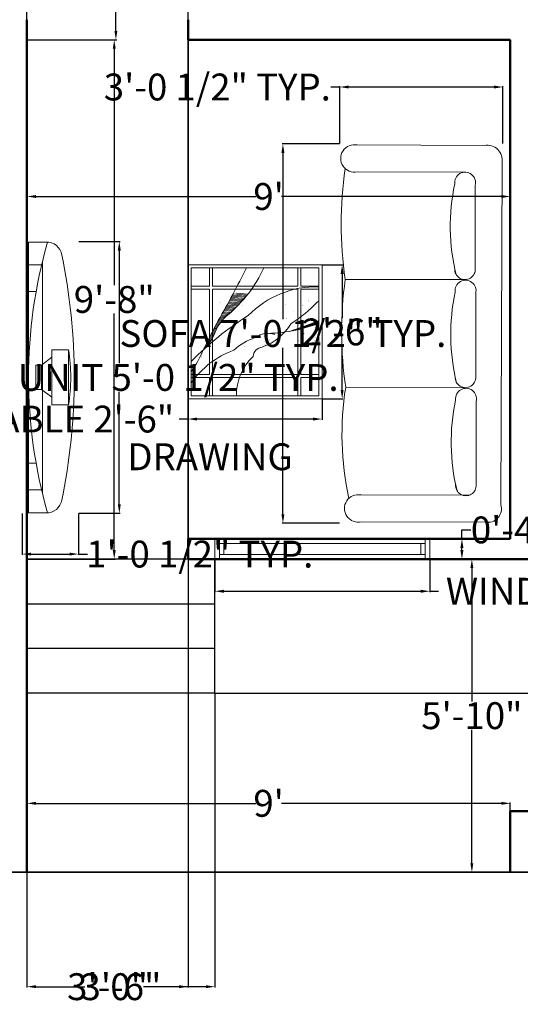
# Model space of a CAD drawing. Units: inches. Extents: x 134 to 568, y 15 to 554.
# Tile 2 of 7: x 303 to 415, y 15 to 235. Entities that reach past the tile are written whole.
import ezdxf

# ---------------------------------------------------------------- set-up
doc = ezdxf.new("R2010")
doc.units = ezdxf.units.IN
doc.header["$MEASUREMENT"] = 0
for name, color, linetype, lineweight in [('A-ANNO-DIMS', 2, 'Continuous', 18), ('A-AREA-IDEN', 7, 'Continuous', 25), ('A-EQPM', 8, 'Continuous', 18), ('A-FLOR-STRS', 3, 'Continuous', 25), ('A-FURN', 9, 'Continuous', 18), ('A-GLAZ', 4, 'Continuous', 18), ('A-WALL', 7, 'Continuous', 50), ('C-PROP', 7, 'Continuous', 35)]:
    doc.layers.add(name, color=color, linetype=linetype, lineweight=lineweight)
doc.styles.get("Standard").update_dxf_attribs({"font": 'arial.ttf'})
doc.dimstyles.get("Standard").update_dxf_attribs({"dimtxt": 6, "dimasz": 2, "dimexe": 0.18, "dimexo": 0.0625, "dimgap": 0.09, "dimtad": 0, "dimtih": 1, "dimtoh": 1, "dimdec": 0, "dimzin": 0, "dimdsep": 46, "dimlunit": 4, "dimtxsty": 'Standard', "dimcen": 0.09, "dimadec": 0, "dimazin": 0, "dimtfac": 1, "dimtdec": 0, "dimtofl": 0, "dimtmove": 0, "dimatfit": 3, "dimfxl": 1, "dimtolj": 1, "dimtzin": 0, "dimarcsym": 0})

# ---------------------------------------------------------------- blocks, each defined once
blk = doc.blocks.new('window 4.5')
for p, q in [((346.5833573093669, -32.94169834523767), (346.5833573093669, -28.44169834523766)), ((346.5833573093669, -28.44169834523766), (394.5833573093669, -28.44169834523766)), ((347.5833573093669, -32.94169834523768), (347.583357309367, -28.44169834523767)), ((393.5833573093669, -28.44169834523766), (393.5833573093669, -32.94169834523766)), ((394.5833573093669, -28.44169834523766), (394.5833573093669, -32.94169834523766)), ((347.5833573093669, -29.44169834523766), (393.5833573093669, -29.44169834523765)), ((348.5833573093669, -31.94169834523767), (348.5833573093669, -29.44169834523765)), ((392.5833573093669, -29.44169834523765), (392.5833573093669, -31.94169834523766)), ((394.5833573093669, -32.94169834523766), (346.5833573093669, -32.94169834523767)), ((393.5833573093669, -31.94169834523766), (347.5833573093669, -31.94169834523767))]:
    blk.add_line(p, q)
blk = doc.blocks.new('*D10')
at = {"layer": 'A-ANNO-DIMS', "color": 0, "lineweight": -2, "transparency": 16777216}
for p, q in [((304.583357309367, 44.64466191446035), (304.583357309367, 60.17594326257374)), ((306.583357309367, 59.99594326257374), (355.7327843216453, 59.99594326257374)), ((410.5833573093669, 59.99594326257374), (361.4339302970887, 59.99594326257374)), ((412.583357309367, 44.64466191446035), (412.583357309367, 60.17594326257374))]:
    blk.add_line(p, q, dxfattribs=at)
at = {"layer": 'A-ANNO-DIMS', "color": 0, "transparency": 16777216}
for points in [[(306.583357309367, 60.32927659590708), (306.583357309367, 59.66260992924041), (304.583357309367, 59.99594326257374)], [(410.5833573093669, 60.32927659590708), (410.5833573093669, 59.66260992924041), (412.583357309367, 59.99594326257374)]]:
    blk.add_solid(points, dxfattribs=at)
at = {"layer": 'Defpoints', "color": 0, "transparency": 16777216}
for p in [(412.583357309367, 59.99594326257374), (304.583357309367, 44.58216191446036), (412.583357309367, 44.58216191446036)]:
    blk.add_point(p, dxfattribs=at)
at = {"layer": 'A-ANNO-DIMS', "color": 0, "transparency": 16777216, "insert": (358.583357309367, 59.99594326257374), "char_height": 6, "attachment_point": 5}
blk.add_mtext("\\A1;9'", dxfattribs=at)
blk = doc.blocks.new('*D11')
at = {"layer": 'A-ANNO-DIMS', "color": 0, "lineweight": -2, "transparency": 16777216}
for p, q in [((417.020857309367, 114.5821619144604), (403.8256208830564, 114.5821619144604)), ((404.0056208830565, 112.5821619144604), (404.0056208830565, 82.73559984079056)), ((404.0056208830565, 46.58216191446037), (404.0056208830565, 76.42872398813023)), ((412.5208573093671, 44.58216191446036), (403.8256208830564, 44.58216191446036))]:
    blk.add_line(p, q, dxfattribs=at)
at = {"layer": 'A-ANNO-DIMS', "color": 0, "transparency": 16777216}
for points in [[(403.6722875497232, 112.5821619144604), (404.3389542163898, 112.5821619144604), (404.0056208830565, 114.5821619144604)], [(403.6722875497232, 46.58216191446037), (404.3389542163898, 46.58216191446037), (404.0056208830565, 44.58216191446036)]]:
    blk.add_solid(points, dxfattribs=at)
at = {"layer": 'Defpoints', "color": 0, "transparency": 16777216}
for p in [(404.0056208830565, 114.5821619144604), (417.0833573093671, 114.5821619144604), (412.5833573093671, 44.58216191446036)]:
    blk.add_point(p, dxfattribs=at)
at = {"layer": 'A-ANNO-DIMS', "color": 0, "transparency": 16777216, "insert": (404.0056208830564, 79.58216191446026), "char_height": 6, "attachment_point": 5}
blk.add_mtext('\\A1;5\'-10"', dxfattribs=at)
blk = doc.blocks.new('*D12')
at = {"layer": 'A-ANNO-DIMS', "color": 0, "lineweight": -2, "transparency": 16777216}
for p, q in [((304.5833573093669, 230.5196619144604), (304.5833573093669, 195.3989397718649)), ((412.5833573093668, 230.5196619144604), (412.5833573093668, 195.3989397718649)), ((306.5833573093669, 195.5789397718649), (355.7327843216452, 195.5789397718649)), ((410.5833573093669, 195.5789397718649), (361.4339302970886, 195.5789397718649))]:
    blk.add_line(p, q, dxfattribs=at)
at = {"layer": 'A-ANNO-DIMS', "color": 0, "transparency": 16777216}
for points in [[(306.5833573093669, 195.9122731051983), (306.5833573093669, 195.2456064385316), (304.5833573093669, 195.5789397718649)], [(410.5833573093669, 195.9122731051983), (410.5833573093669, 195.2456064385316), (412.5833573093668, 195.5789397718649)]]:
    blk.add_solid(points, dxfattribs=at)
at = {"layer": 'Defpoints', "color": 0, "transparency": 16777216}
for p in [(304.5833573093669, 230.5821619144603), (412.5833573093668, 230.5821619144603), (412.5833573093668, 195.5789397718649)]:
    blk.add_point(p, dxfattribs=at)
at = {"layer": 'A-ANNO-DIMS', "color": 0, "transparency": 16777216, "insert": (358.5833573093669, 195.5789397718649), "char_height": 6, "attachment_point": 5}
blk.add_mtext("\\A1;9'", dxfattribs=at)
blk = doc.blocks.new('*D13')
at = {"layer": 'A-ANNO-DIMS', "color": 0, "lineweight": -2, "transparency": 16777216}
for p, q in [((304.6458573093671, 230.5821619144605), (324.2629623244103, 230.5821619144605)), ((324.0829623244104, 228.5821619144605), (324.0829623244104, 175.7355998407906)), ((324.0829623244104, 116.5821619144604), (324.0829623244104, 169.4287239881303)), ((304.6458573093671, 114.5821619144604), (324.2629623244104, 114.5821619144604))]:
    blk.add_line(p, q, dxfattribs=at)
at = {"layer": 'A-ANNO-DIMS', "color": 0, "transparency": 16777216}
for points in [[(323.749628991077, 228.5821619144605), (324.4162956577437, 228.5821619144605), (324.0829623244104, 230.5821619144605)], [(323.7496289910771, 116.5821619144604), (324.4162956577437, 116.5821619144604), (324.0829623244104, 114.5821619144604)]]:
    blk.add_solid(points, dxfattribs=at)
at = {"layer": 'Defpoints', "color": 0, "transparency": 16777216}
for p in [(304.583357309367, 230.5821619144605), (324.0829623244104, 230.5821619144605), (304.5833573093671, 114.5821619144604)]:
    blk.add_point(p, dxfattribs=at)
at = {"layer": 'A-ANNO-DIMS', "color": 0, "transparency": 16777216, "insert": (324.0829623244104, 172.5821619144603), "char_height": 6, "attachment_point": 5}
blk.add_mtext('\\A1;9\'-8"', dxfattribs=at)
blk = doc.blocks.new('*D23')
at = {"layer": 'A-ANNO-DIMS', "color": 0, "lineweight": -2, "transparency": 16777216}
for p, q in [((316.645857309367, 367.0821619144605), (324.6429623244108, 367.0821619144605)), ((324.4629623244108, 365.0821619144605), (324.4629623244108, 301.9344402227825)), ((324.4629623244108, 232.5821619144606), (324.4629623244108, 295.7298836061386)), ((324.1454623244103, 230.5821619144606), (324.6429623244108, 230.5821619144606))]:
    blk.add_line(p, q, dxfattribs=at)
at = {"layer": 'A-ANNO-DIMS', "color": 0, "transparency": 16777216}
for points in [[(324.1296289910775, 365.0821619144605), (324.7962956577441, 365.0821619144605), (324.4629623244108, 367.0821619144605)], [(324.1296289910775, 232.5821619144606), (324.7962956577441, 232.5821619144606), (324.4629623244108, 230.5821619144606)]]:
    blk.add_solid(points, dxfattribs=at)
at = {"layer": 'Defpoints', "color": 0, "transparency": 16777216}
for p in [(316.583357309367, 367.0821619144605), (324.0829623244102, 230.5821619144606), (324.4629623244108, 230.5821619144606)]:
    blk.add_point(p, dxfattribs=at)
at = {"layer": 'A-ANNO-DIMS', "color": 0, "transparency": 16777216, "insert": (324.4629623244108, 298.8321619144604), "char_height": 6, "attachment_point": 5}
blk.add_mtext("\\A1;11'", dxfattribs=at)
blk = doc.blocks.new('A$C78AE5658')
for p, q in [((1514.710072450669, 306.1060037219359), (1514.710072450669, 524.1059474034627)), ((1514.710072450669, 524.1059474034627), (2235.5102586675, 524.1059474034627)), ((2235.5102586675, 306.1060037219359), (2235.5102586675, 524.1059474034627)), ((1514.710072450669, 306.1060037219359), (2235.5102586675, 306.1060037219359)), ((1613.280102290542, 306.1060037219359), (1715.729798347087, 167.9763742110153)), ((2136.940228827627, 306.1060037219359), (2034.490532771082, 167.9763742110153)), ((98.35715676363363, 250.0000009555879), (98.35715676363363, 251.6199660723724)), ((98.35715676367727, 250.0000009555733), (98.35715676361907, 9.555878933e-07)), ((348.3571567636482, 183.569161564541), (3398.357156763547, 183.5691615645264)), ((398.3571567636482, 9.555733413e-07), (398.3571567636482, 171.5666306721468)), ((2034.490532771082, 167.9763742110153), (1715.729425914915, 167.9763742110153)), ((1715.729425914915, 167.9763742110153), (1715.729425914915, 97.54311758768019)), ((2034.490532771082, 167.9763742110153), (2034.490532771082, 97.54311758768019)), ((3348.35715676359, 9.555733413e-07), (3348.35715676359, 171.5666306721468)), ((3648.35715676359, 250.0000009555733), (3648.35715676359, 251.6199660720231)), ((3648.35715676359, 9.555733413e-07), (3648.35715676359, 250.0000009555733)), ((3648.357156763605, 9.555733413e-07), (98.35715676363363, 9.555878933e-07)), ((748.357156763648, 9.555733413e-07), (748.357156763648, 99.2393274621354)), ((2034.490532771082, 97.54311758768019), (1715.729425914915, 97.54311758768019)), ((2998.35715676359, 9.555733413e-07), (2998.35715676359, 99.2393274621354))]:
    blk.add_line(p, q)
blk.add_lwpolyline([(246.4015375078543, 431.9827464358895, -0.103184122095167), (3500.312775983877, 431.9827464432965, -0.103184122095167)], format="xyb")
for centre, radius, start, end in [((1875.110165559085, -1674.917347937364), 2228.360760865037, 80.69248372113285, 99.30751627886714), ((297.9418522906435, 238.7378345952966), 200, 98.46874505780073, 183.6930153877844), ((3448.772461236565, 238.7378345952966), 200, 356.3069846122155, 81.53125494219925), ((1873.357156763633, 6426.250000955618), 6426.25000000003, 253.9658138527447, 286.0341861472553)]:
    blk.add_arc(centre, radius, start, end)
blk = doc.blocks.new('A$C25EC1EFB')
h = blk.add_hatch()
h.set_pattern_fill('ANSI31', color=256, scale=2.508, angle=580, style=0)
h.set_pattern_definition([(94.99999999999984, (2801.512250582819, 4289.79602251789), (7.93259876143476, 0.6940124639253284), [])])
edge = h.paths.add_edge_path()
edge.add_ellipse((4084.490467177063, -2815.580363917667), major_axis=(-3872.16408689083, 3872.16408689083), ratio=0.9999999999995552, start_angle=340.89961915580596, end_angle=343.15488567038426, ccw=False)
edge.add_ellipse((1486.624568246823, 2293.159848771007), major_axis=(-194.6618757392838, 194.6618757392838), ratio=0.9999999999999246, start_angle=154.9056197196584, end_angle=183.4247301497222, ccw=False)
edge.add_ellipse((1687.117678346121, 1762.501521206774), major_axis=(-206.4950185728816, 206.4950185728816), ratio=0.999999999999898, start_angle=-23.5559095241906, end_angle=5.886608761987814)
edge.add_ellipse((823.8605303866296, 2467.162105106873), major_axis=(-581.4647167234576, 581.4647167234575), ratio=0.9999999999998493, start_angle=171.3363574034995, end_angle=185.7365630084011, ccw=False)
edge.add_line((1311.102457978037, 1804.744006331188), (1311.102457978037, 1908.515397835807))
edge.add_ellipse((-1407.416444189095, 7084.924681207201), major_axis=(4134.341428234145, 4134.341428234145), ratio=0.9999999999998351, start_angle=252.7073165240117, end_angle=254.8255249662156)
for p, q in [((1118.231915589249, 2219.932055225661), (1118.231915589242, 1300.332055225655)), ((2037.831915589246, 2219.932055225647), (1118.231915589249, 2219.932055225661)), ((2016.931915589244, 2199.032055225638), (1139.131915589243, 2199.032055225638)), ((1139.131915589243, 2199.032055225638), (1139.131915589243, 1321.232055225664)), ((1264.531915589245, 2199.032055225638), (1264.531915589245, 2073.63205522563)), ((1285.431915589246, 2199.032055225638), (1285.431915589246, 2073.63205522563)), ((1870.631915589243, 2199.032055225638), (1870.631915589243, 2073.632055225644)), ((1891.531915589245, 2199.032055225638), (1891.531915589245, 2073.632055225644)), ((2016.931915589244, 2199.032055225638), (2016.931915589244, 1321.23205522565)), ((2037.831915589246, 2219.932055225647), (2037.831915589246, 1300.332055225655)), ((1264.531915589245, 2073.63205522563), (1139.131915589243, 2073.632055225644)), ((1264.531915589245, 2052.732055225635), (1139.131915589243, 2052.732055225664)), ((1264.531915589245, 2052.732055225635), (1264.531915589245, 1467.532055225652)), ((1870.631915589243, 2073.632055225644), (1285.431915589246, 2073.63205522563)), ((1870.631915589243, 2052.73205522565), (1285.431915589246, 2052.732055225635)), ((1285.431915589246, 2052.732055225635), (1285.431915589246, 1467.532055225652)), ((1870.631915589243, 2052.73205522565), (1870.631915589243, 1467.532055225652)), ((2016.931915589244, 2073.632055225658), (1891.531915589245, 2073.632055225644)), ((1891.531915589245, 2052.73205522565), (1891.531915589245, 1467.532055225652)), ((2016.931915589244, 2052.73205522565), (1891.531915589245, 2052.73205522565)), ((1565.849127400865, 1480.689699283357), (1564.688483608976, 1493.955918529544)), ((1569.58961247749, 1498.845113355761), (1568.886649074042, 1506.88002182413)), ((1573.215999468995, 1518.30467450877), (1573.064505181503, 1520.03626213839)), ((1264.531915589245, 1467.532055225667), (1139.131915589243, 1467.532055225667)), ((1264.531915589245, 1446.632055225658), (1139.131915589243, 1446.632055225658)), ((1264.531915589245, 1446.632055225658), (1264.531915589245, 1321.23205522565)), ((1870.631915589243, 1467.532055225652), (1285.431915589246, 1467.532055225667)), ((1870.631915589243, 1446.632055225658), (1285.431915589246, 1446.632055225658)), ((1285.431915589246, 1446.632055225658), (1285.431915589246, 1321.23205522565)), ((1541.818491434993, 1389.905000426101), (1539.119938526573, 1420.749601311116)), ((1545.9666700701, 1403.400455801595), (1543.422872825396, 1432.476191356145)), ((1550.066663663807, 1417.446668720506), (1547.710096352946, 1444.382356338588)), ((1554.112776362645, 1432.108743085911), (1551.980974986758, 1456.475344311409)), ((1558.098049746682, 1447.466214001491), (1556.234828786708, 1468.762927025651)), ((1562.013830635669, 1463.617987770158), (1560.470927201475, 1481.253454721161)), ((1870.631915589243, 1446.632055225658), (1870.631915589243, 1321.23205522565)), ((2016.931915589244, 1467.532055225652), (1891.531915589245, 1467.532055225652)), ((1891.531915589245, 1446.632055225658), (1891.531915589245, 1321.23205522565)), ((2016.931915589244, 1446.632055225658), (1891.531915589245, 1446.632055225658)), ((1515.85332769347, 1321.232055225664), (1513.003113907138, 1353.810147877557)), ((1520.497301609701, 1329.060544606509), (1517.389086063931, 1364.587610862924)), ((1524.828260129872, 1340.466816335822), (1521.762395858635, 1375.50980530923)), ((1529.128590691436, 1352.223167233933), (1526.122610320157, 1386.58168009873)), ((1533.395763262031, 1364.358515703112), (1530.469269874078, 1397.808488191054)), ((1537.626860969483, 1376.906201744794), (1534.801885985626, 1409.195813564198)), ((2037.831915589246, 1300.332055225655), (1118.231915589242, 1300.332055225655)), ((2016.931915589244, 1321.23205522565), (1139.131915589243, 1321.232055225664)), ((1499.866693724727, 1321.232055225664), (1499.773196894175, 1322.300728889044)), ((1505.195571714308, 1321.23205522565), (1504.194793856486, 1332.670998484005)), ((1510.524449703889, 1321.232055225664), (1508.604887871583, 1343.172747367374))]:
    blk.add_line(p, q)
at = {"const_width": 2.09}
for points in [[(1511.151005801041, 2155.427417849518, -1), (1511.151005801041, 2153.337417849522, -1)], [(1749.963977974703, 2129.419879811459, -1), (1749.963977974703, 2127.329879811463, -1)], [(1378.464403896922, 2001.982938292022, -1), (1378.464403896922, 1999.892938292025, -1)], [(1378.464403896922, 2000.937938292024, -1), (1378.464403896922, 1998.847938292026, -1)], [(1472.141222166467, 1950.101574691951, -1), (1472.141222166467, 1948.011574691955, -1)], [(1498.485842016862, 1893.112440112549, -1), (1498.485842016862, 1891.022440112552, -1)], [(1589.664228032883, 1926.272639169089, -1), (1589.664228032883, 1924.182639169077, -1)], [(1396.649697045645, 1848.538458734525, -1), (1396.649697045645, 1846.448458734528, -1)], [(1677.799055322533, 1835.246250902906, -1), (1677.799055322533, 1833.15625090291, -1)], [(1661.635412078192, 1692.493220240234, -1), (1661.635412078192, 1690.403220240223, -1)], [(1682.418605074026, 1710.698501999875, -1), (1682.418605074026, 1708.608501999864, -1)], [(1632.519993189891, 1660.01154033171, -1), (1632.519993189891, 1657.921540331714, -1)], [(1672.027005685611, 1645.679651771737, -1), (1672.027005685611, 1643.589651771741, -1)], [(1390.689109610934, 1549.797216376151, -1), (1390.689109610934, 1547.707216376155, -1)], [(1435.398901256181, 1495.038386561347, -1), (1435.398901256181, 1492.948386561351, -1)], [(1484.978268723158, 1546.850996961155, -1), (1484.978268723158, 1544.760996961158, -1)], [(1519.878047569999, 1513.762184183615, -1), (1519.878047569999, 1511.672184183619, -1)], [(1394.744337709578, 1434.839303017281, -1), (1394.744337709578, 1432.74930301727, -1)], [(1587.165183262217, 1425.04444594484, -1), (1587.165183262217, 1422.954445944844, -1)], [(1638.254319235255, 1463.626875239402, -1), (1638.254319235255, 1461.536875239391, -1)], [(1675.222175186443, 1421.779486743347, -1), (1675.222175186443, 1419.689486743351, -1)], [(1675.788258493603, 1422.657879986356, -1), (1675.788258493603, 1420.567879986345, -1)], [(1365.392005141164, 1392.394905260015, -1), (1365.392005141164, 1390.304905260018, -1)], [(1639.675595830262, 1353.891867756152, -1), (1639.675595830262, 1351.801867756156, -1)], [(1370.896625781812, 1333.067117625229, -1), (1370.896625781812, 1330.977117625232, -1)], [(1613.584636758898, 1347.361959619193, -1), (1613.584636758898, 1345.271959619196, -1)]]:
    blk.add_lwpolyline(points, format="xyb", close=True, dxfattribs=at)
for centre, radius, start, end in [((3333.68451552435, 627.3607967675852), 2209.54164879086, 134.6725360764692, 147.7436105193565), ((2287.848786312694, 1688.392912899486), 624.2670274309789, 125.1781643370384, 159.5766212149076), ((1462.653166443046, 2709.567626046374), 640.2705249755662, 292.8904712152515, 307.0626715443762), ((4084.490467176721, -2815.580363917798), 5476.066967415318, 115.6772969660199, 118.1548856704495), ((1486.624568246801, 2293.159848771022), 275.2934647474958, 289.9056197197872, 318.4247301496573), ((1687.117678346143, 1762.501521206774), 292.0280558282651, 111.4440904757719, 140.8866087620124), ((-2476.242387987366, 8989.86383017015), 8031.077363206627, 296.7547849003873, 299.6814985470403), ((751.7750952702208, 2534.062472635524), 920.4881034674244, 294.8861636343854, 320.3521788954757), ((2051.740526511305, 1602.642054351665), 462.5051862275705, 138.9735804164881, 160.2295429731453), ((2014.166362558564, 1518.116840648719), 370.3125627779616, 89.60713639418466, 136.3509345096815), ((1916.655318256047, 1341.313739382756), 648.3552410927683, 134.1383379809644, 181.6847040310653), ((1726.67177394053, 1673.301525916809), 139.6326613666137, 142.0948538523169, 200.8895128689712), ((1752.222980010354, 1704.369846744921), 69.61106324809847, 94.95105755802923, 174.8766543317414), ((576.7142338831854, 1693.940106953196), 1011.861440092256, 338.386783207812, 0.0010917430398909), ((1322.831429736014, 1838.987718223034), 381.1559142689087, 301.1293017828129, 340.1644872338225), ((792.9020607460498, 1960.337764563381), 853.7319657820956, 312.6112985239825, 328.3781661717325), ((-408.4163850434979, 2142.027900565321), 2076.810081976653, 336.7203354898851, 342.6666348099279), ((1307.752931048004, 1350.181809599417), 65.70312471435534, 333.8568999860387, 343.9551289370007)]:
    blk.add_arc(centre, radius, start, end)
blk = doc.blocks.new('SOFA-3-SEAT')
for p, q in [((2.639539900301173, 84.33324550660927, -275.7706107739931), (31.48293072343935, 84.25018466807978, -275.7706107739931)), ((0.0383790449484991, 3.974159020291153, -275.7706107739931), (0.3339295813419483, 80.44811578913232, -275.7706107739931)), ((7.498200915528144, 78.33324550660927, -275.7706107739931), (31.56791808250259, 78.25018466807978, -275.7706107739931)), ((5.843710623688679, 57.34215320189196, -275.7706107739931), (5.843710623688679, 75.93023828611786, -275.7706107739931)), ((5.843710623688679, 57.34215320189196, -275.7706107739931), (5.843710623688679, 75.93023828611786, -275.7706107739931)), ((34.99945515191198, 54.21758312230394, -275.7706107739931), (8.231751979335826, 54.28260851868344, -275.7706107739931)), ((5.943773992104809, 33.20240762962658, -275.7706107739931), (5.943773992104837, 51.79049271384883, -275.7706107739931)), ((5.943773992104809, 33.20240762962658, -275.7706107739931), (5.943773992104837, 51.79049271385611, -275.7706107739931)), ((35.09951852032811, 30.07783755003129, -275.7706107739931), (8.331815347751956, 30.14286294641079, -275.7706107739931)), ((6.043837360520967, 9.062662057353918, -275.7706107739931), (6.043837360520967, 27.65074714157618, -275.7706107739931)), ((6.043837360520967, 9.062662057353918, -275.7706107739931), (6.043837360520967, 27.65074714157618, -275.7706107739931)), ((8.302397746832696, 6.142582730023605, -275.7706107739931), (32.4491326919013, 6.059521891490476, -275.7706107739931)), ((3.975506222290107, 0.1425827300236051, -275.7706107739931), (32.4491326919013, 0.0595218914904763, -275.7706107739931))]:
    blk.add_line(p, q)
for centre, radius, start, end in [((3.220976162505252, 81.35906493094171, -275.7706107739931), 3.02735301884233, 78.91083061777086, 197.5120367194869), ((32.20255676183283, 81.25977594989763, -275.7706107739931), 3.075777289872148, 258.0923749518217, 103.5306555133332), ((8.131688610919667, 76.12601528668618, -275.7706107739931), 2.296338804262066, 355.1092454701771, 184.8907545298229), ((-33.55016406365772, 66.49239086433681, -275.7706107739931), 44.97131277140765, 347.8856334289421, 13.9133261029634), ((-31.3836276940348, 64.73871829630025, -275.7706107739931), 67.21166545684105, 350.9940323093792, 12.25610082943838), ((8.103939744214443, 56.75685568044809, -275.7706107739931), 2.334782402231908, 165.4818835729592, 7.325225020201399), ((8.231751979335826, 51.98626971442445, -275.7706107739931), 2.296338804262066, 355.1092454701771, 184.8907545298229), ((-33.45010069524156, 42.35264529206415, -275.7706107739931), 44.97131277140765, 347.8856334289421, 13.9133261029634), ((-49.15139397142789, 41.79868330390036, -275.7706107739931), 85.06229764636532, 352.0799408120631, 8.39505804799601), ((8.204003112630573, 32.61711010817544, -275.7706107739931), 2.334782402231908, 165.4818835729592, 7.325225020201399), ((8.331815347751956, 27.84652414215179, -275.7706107739931), 2.296338804262066, 355.1092454701771, 184.8907545298229), ((-33.3500373268254, 18.21289971979877, -275.7706107739931), 44.97131277140765, 347.8856334289421, 13.9133261029634), ((-49.05133060301174, 17.65893773163134, -275.7706107739931), 85.06229764636532, 351.661265989887, 8.39505804799601), ((8.304066481017628, 8.477364535906418, -275.7706107739931), 2.334782402231908, 165.4818835729592, 7.325225020201399), ((33.05221387278999, 3.059521891490476, -275.7706107739931), 3.060017469021007, 258.6334958280249, 101.366504171975), ((3.371955953108965, 3.460987091163588, -275.7706107739931), 3.37284456082161, 171.2485666807343, 280.3082563582749)]:
    blk.add_arc(centre, radius, start, end)
blk = doc.blocks.new('*D38')
at = {"layer": 'A-ANNO-DIMS', "color": 0, "lineweight": -2, "transparency": 16777216}
for p, q in [((316.172408782906, 185.5132349532936), (325.3973721430653, 185.5132349532937)), ((325.2173721430653, 183.5132349532937), (325.2173721430653, 158.3473429887794)), ((325.2173721430653, 126.7968125522324), (325.2173721430653, 151.9627045167466)), ((316.172408782906, 124.7968125522324), (325.3973721430654, 124.7968125522324))]:
    blk.add_line(p, q, dxfattribs=at)
at = {"layer": 'A-ANNO-DIMS', "color": 0, "transparency": 16777216}
for points in [[(324.884038809732, 183.5132349532937), (325.5507054763986, 183.5132349532937), (325.2173721430653, 185.5132349532937)], [(324.884038809732, 126.7968125522324), (325.5507054763987, 126.7968125522324), (325.2173721430653, 124.7968125522324)]]:
    blk.add_solid(points, dxfattribs=at)
at = {"layer": 'Defpoints', "color": 0, "transparency": 16777216}
for p in [(316.109908782906, 185.5132349532936), (325.2173721430653, 185.5132349532937), (316.109908782906, 124.7968125522324)]:
    blk.add_point(p, dxfattribs=at)
at = {"layer": 'A-ANNO-DIMS', "color": 0, "transparency": 16777216, "insert": (325.2173721430653, 155.1550237527629), "char_height": 6, "attachment_point": 5}
blk.add_mtext('\\A1;MEDIA UNIT 5\'-0 1/2" TYP.', dxfattribs=at)
blk = doc.blocks.new('*D39')
at = {"layer": 'A-ANNO-DIMS', "color": 0, "lineweight": -2, "transparency": 16777216}
for p, q in [((303.515583724388, 124.7343125522323), (303.515583724388, 115.5093491920731)), ((316.1099087829058, 124.7343125522323), (316.1099087829058, 115.5093491920731)), ((305.515583724388, 115.6893491920731), (314.1099087829058, 115.6893491920731)), ((316.1099087829058, 115.6893491920731), (318.1099087829058, 115.6893491920731))]:
    blk.add_line(p, q, dxfattribs=at)
at = {"layer": 'A-ANNO-DIMS', "color": 0, "transparency": 16777216}
for points in [[(305.515583724388, 116.0226825254064), (305.515583724388, 115.3560158587398), (303.515583724388, 115.6893491920731)], [(314.1099087829058, 116.0226825254064), (314.1099087829058, 115.3560158587398), (316.1099087829058, 115.6893491920731)]]:
    blk.add_solid(points, dxfattribs=at)
at = {"layer": 'Defpoints', "color": 0, "transparency": 16777216}
for p in [(303.515583724388, 124.7968125522323), (316.1099087829058, 124.7968125522323), (316.1099087829058, 115.6893491920731)]:
    blk.add_point(p, dxfattribs=at)
at = {"layer": 'A-ANNO-DIMS', "color": 0, "transparency": 16777216, "insert": (343.194451756985, 115.6893491920731), "char_height": 6, "attachment_point": 5}
blk.add_mtext('\\A1;1\'-0 1/2" TYP.', dxfattribs=at)
blk = doc.blocks.new('*D44')
at = {"layer": 'A-ANNO-DIMS', "color": 0, "lineweight": -2, "transparency": 16777216}
for p, q in [((374.4263709433948, 207.3322603239445), (361.5993065679185, 207.3322603239445)), ((361.7793065679185, 205.3322603239445), (361.7793065679185, 168.1614113597598)), ((361.7793065679186, 124.6018311541018), (361.7793065679185, 161.7726801182864)), ((374.4263709433948, 122.6018311541018), (361.5993065679186, 122.6018311541018))]:
    blk.add_line(p, q, dxfattribs=at)
at = {"layer": 'A-ANNO-DIMS', "color": 0, "transparency": 16777216}
for points in [[(361.4459732345852, 205.3322603239445), (362.1126399012518, 205.3322603239445), (361.7793065679185, 207.3322603239445)], [(361.4459732345853, 124.6018311541018), (362.1126399012519, 124.6018311541018), (361.7793065679186, 122.6018311541018)]]:
    blk.add_solid(points, dxfattribs=at)
at = {"layer": 'Defpoints', "color": 0, "transparency": 16777216}
for p in [(374.4888709433948, 207.3322603239445), (361.7793065679186, 122.6018311541018), (374.4888709433948, 122.6018311541018)]:
    blk.add_point(p, dxfattribs=at)
at = {"layer": 'A-ANNO-DIMS', "color": 0, "transparency": 16777216, "insert": (361.7793065679185, 164.967045739023), "char_height": 6, "attachment_point": 5}
blk.add_mtext('\\A1;SOFA 7\'-0 1/2" TYP.', dxfattribs=at)
blk = doc.blocks.new('*D45')
at = {"layer": 'A-ANNO-DIMS', "color": 0, "lineweight": -2, "transparency": 16777216}
for p, q in [((374.4888709433947, 220.0418246994208), (372.4888709433947, 220.0418246994208)), ((374.4888709433947, 207.3947603239444), (374.4888709433947, 220.2218246994208)), ((408.9312259875706, 220.0418246994208), (376.4888709433947, 220.0418246994208)), ((410.9312259875706, 207.3947603239444), (410.9312259875706, 220.2218246994208))]:
    blk.add_line(p, q, dxfattribs=at)
at = {"layer": 'A-ANNO-DIMS', "color": 0, "transparency": 16777216}
for points in [[(376.4888709433947, 220.3751580327542), (376.4888709433947, 219.7084913660875), (374.4888709433947, 220.0418246994208)], [(408.9312259875706, 220.3751580327542), (408.9312259875706, 219.7084913660875), (410.9312259875706, 220.0418246994208)]]:
    blk.add_solid(points, dxfattribs=at)
at = {"layer": 'Defpoints', "color": 0, "transparency": 16777216}
for p in [(374.4888709433947, 220.0418246994208), (374.4888709433947, 207.3322603239444), (410.9312259875706, 207.3322603239444)]:
    blk.add_point(p, dxfattribs=at)
at = {"layer": 'A-ANNO-DIMS', "color": 0, "transparency": 16777216, "insert": (347.1239732626307, 220.0418246994208), "char_height": 6, "attachment_point": 5}
blk.add_mtext('\\A1;3\'-0 1/2" TYP.', dxfattribs=at)
blk = doc.blocks.new('*D48')
at = {"layer": 'A-ANNO-DIMS', "color": 0, "lineweight": -2, "transparency": 16777216}
for p, q in [((340.5750090510671, 150.2827316451021), (340.5750090510671, 145.672982833064)), ((370.523334464654, 150.2827316451021), (370.523334464654, 145.672982833064)), ((340.5750090510671, 145.852982833064), (338.5750090510671, 145.852982833064)), ((368.523334464654, 145.852982833064), (342.5750090510671, 145.852982833064))]:
    blk.add_line(p, q, dxfattribs=at)
at = {"layer": 'A-ANNO-DIMS', "color": 0, "transparency": 16777216}
for points in [[(342.5750090510671, 146.1863161663974), (342.5750090510671, 145.5196494997307), (340.5750090510671, 145.852982833064)], [(368.523334464654, 146.1863161663974), (368.523334464654, 145.5196494997307), (370.523334464654, 145.852982833064)]]:
    blk.add_solid(points, dxfattribs=at)
at = {"layer": 'Defpoints', "color": 0, "transparency": 16777216}
for p in [(340.5750090510671, 150.3452316451021), (370.523334464654, 150.3452316451021), (340.5750090510671, 145.852982833064)]:
    blk.add_point(p, dxfattribs=at)
at = {"layer": 'A-ANNO-DIMS', "color": 0, "transparency": 16777216, "insert": (305.4911482052281, 145.852982833064), "char_height": 6, "attachment_point": 5}
blk.add_mtext('\\A1;LOW TABLE 2\'-6"', dxfattribs=at)
blk = doc.blocks.new('*D49')
at = {"layer": 'A-ANNO-DIMS', "color": 0, "lineweight": -2, "transparency": 16777216}
for p, q in [((370.5858344646541, 180.2935570586889), (375.1955832766922, 180.2935570586889)), ((375.0155832766922, 178.293557058689), (375.0155832766922, 168.4728322782257)), ((375.0155832766922, 152.3452316451021), (375.0155832766922, 162.1659564255654)), ((370.5858344646541, 150.3452316451021), (375.1955832766922, 150.3452316451021))]:
    blk.add_line(p, q, dxfattribs=at)
at = {"layer": 'A-ANNO-DIMS', "color": 0, "transparency": 16777216}
for points in [[(374.6822499433589, 178.293557058689), (375.3489166100255, 178.293557058689), (375.0155832766922, 180.2935570586889)], [(374.6822499433589, 152.3452316451021), (375.3489166100255, 152.3452316451021), (375.0155832766922, 150.3452316451021)]]:
    blk.add_solid(points, dxfattribs=at)
at = {"layer": 'Defpoints', "color": 0, "transparency": 16777216}
for p in [(370.5233344646541, 180.2935570586889), (370.5233344646541, 150.3452316451021), (375.0155832766922, 150.3452316451021)]:
    blk.add_point(p, dxfattribs=at)
at = {"layer": 'A-ANNO-DIMS', "color": 0, "transparency": 16777216, "insert": (375.0155832766922, 165.3193943518954), "char_height": 6, "attachment_point": 5}
blk.add_mtext('\\A1;2\'-6"', dxfattribs=at)
blk = doc.blocks.new('*D50')
at = {"layer": 'A-ANNO-DIMS', "color": 0, "lineweight": -2, "transparency": 16777216}
for p, q in [((346.5833573093669, 114.5196619144603), (346.5833573093669, 107.2021619144603)), ((394.5833573093669, 114.5196619144603), (394.5833573093669, 107.2021619144603)), ((348.5833573093669, 107.3821619144603), (392.5833573093669, 107.3821619144603)), ((394.5833573093669, 107.3821619144603), (396.5833573093669, 107.3821619144603))]:
    blk.add_line(p, q, dxfattribs=at)
at = {"layer": 'A-ANNO-DIMS', "color": 0, "transparency": 16777216}
for points in [[(348.5833573093669, 107.7154952477936), (348.5833573093669, 107.048828581127), (346.5833573093669, 107.3821619144603)], [(392.5833573093669, 107.7154952477936), (392.5833573093669, 107.048828581127), (394.5833573093669, 107.3821619144603)]]:
    blk.add_solid(points, dxfattribs=at)
at = {"layer": 'Defpoints', "color": 0, "transparency": 16777216}
for p in [(346.5833573093669, 114.5821619144603), (394.5833573093669, 114.5821619144603), (394.5833573093669, 107.3821619144603)]:
    blk.add_point(p, dxfattribs=at)
at = {"layer": 'A-ANNO-DIMS', "color": 0, "transparency": 16777216, "insert": (434.6358402561608, 107.3821619144603), "char_height": 6, "attachment_point": 5}
blk.add_mtext('\\A1;WINDOW 4\'-0" TYP.', dxfattribs=at)
blk = doc.blocks.new('*D51')
at = {"layer": 'A-ANNO-DIMS', "color": 0, "lineweight": -2, "transparency": 16777216}
for p, q in [((401.7833573093673, 119.0821619144604), (401.7833573093673, 121.0821619144604)), ((401.7833573093673, 121.0821619144604), (403.7833573093672, 121.0821619144604)), ((394.6458573093671, 119.0821619144604), (401.9633573093673, 119.0821619144604)), ((401.7833573093673, 116.5821619144604), (401.7833573093673, 117.0821619144604)), ((394.6458573093671, 114.5821619144604), (401.9633573093673, 114.5821619144604))]:
    blk.add_line(p, q, dxfattribs=at)
at = {"layer": 'A-ANNO-DIMS', "color": 0, "transparency": 16777216}
for points in [[(401.450023976034, 117.0821619144604), (402.1166906427006, 117.0821619144604), (401.7833573093673, 119.0821619144604)], [(401.450023976034, 116.5821619144604), (402.1166906427006, 116.5821619144604), (401.7833573093673, 114.5821619144604)]]:
    blk.add_solid(points, dxfattribs=at)
at = {"layer": 'Defpoints', "color": 0, "transparency": 16777216}
for p in [(394.5833573093671, 119.0821619144604), (401.7833573093673, 119.0821619144604), (394.5833573093671, 114.5821619144604)]:
    blk.add_point(p, dxfattribs=at)
at = {"layer": 'A-ANNO-DIMS', "color": 0, "transparency": 16777216, "insert": (429.1503013748514, 121.0821619144603), "char_height": 6, "attachment_point": 5}
blk.add_mtext('\\A1;0\'-4 1/2" TYP.', dxfattribs=at)
blk = doc.blocks.new('*D61')
at = {"layer": 'A-ANNO-DIMS', "color": 0, "lineweight": -2, "transparency": 16777216}
for p, q in [((304.583357, 84.519662), (304.583357, 18.85216199999999)), ((346.583357, 84.519662), (346.583357, 18.85216199999999)), ((306.583357, 19.032162), (317.5206421296044, 19.032162)), ((344.583357, 19.032162), (333.6460718703956, 19.032162))]:
    blk.add_line(p, q, dxfattribs=at)
at = {"layer": 'A-ANNO-DIMS', "color": 0, "transparency": 16777216}
for points in [[(306.583357, 19.36549533333333), (306.583357, 18.69882866666667), (304.583357, 19.032162)], [(344.583357, 19.36549533333333), (344.583357, 18.69882866666667), (346.583357, 19.032162)]]:
    blk.add_solid(points, dxfattribs=at)
at = {"layer": 'Defpoints', "color": 0, "transparency": 16777216}
for p in [(304.583357, 84.582162), (346.583357, 84.582162), (346.583357, 19.032162)]:
    blk.add_point(p, dxfattribs=at)
at = {"layer": 'A-ANNO-DIMS', "color": 0, "transparency": 16777216, "insert": (325.583357, 19.032162), "char_height": 6, "attachment_point": 5}
blk.add_mtext('\\A1;3\'-6"', dxfattribs=at)
blk = doc.blocks.new('*D62')
at = {"layer": 'A-ANNO-DIMS', "color": 0, "lineweight": -2, "transparency": 16777216}
for p, q in [((346.6458570000001, 114.582162), (556.8133570000005, 114.5821620000001)), ((556.6333570000004, 112.5821620000001), (556.6333570000004, 102.7355999263302)), ((556.6333570000004, 86.58216200000007), (556.6333570000004, 96.42872407366994)), ((346.6458570000001, 84.58216200000003), (556.8133570000005, 84.58216200000007))]:
    blk.add_line(p, q, dxfattribs=at)
at = {"layer": 'A-ANNO-DIMS', "color": 0, "transparency": 16777216}
for points in [[(556.3000236666671, 112.5821620000001), (556.9666903333338, 112.5821620000001), (556.6333570000004, 114.5821620000001)], [(556.3000236666671, 86.58216200000007), (556.9666903333338, 86.58216200000007), (556.6333570000004, 84.58216200000007)]]:
    blk.add_solid(points, dxfattribs=at)
at = {"layer": 'Defpoints', "color": 0, "transparency": 16777216}
for p in [(346.5833570000001, 114.582162), (556.6333570000004, 114.5821620000001), (346.5833570000001, 84.58216200000003)]:
    blk.add_point(p, dxfattribs=at)
at = {"layer": 'A-ANNO-DIMS', "color": 0, "transparency": 16777216, "insert": (556.6333570000003, 99.5821619999999), "char_height": 6, "attachment_point": 5}
blk.add_mtext('\\A1;2\'-6"', dxfattribs=at)
blk = doc.blocks.new('*D63')
at = {"layer": 'A-ANNO-DIMS', "color": 0, "lineweight": -2, "transparency": 16777216}
for p, q in [((304.583357, 114.644662), (304.583357, 550.312162)), ((306.583357, 550.1321619999999), (314.5206421296044, 550.1321619999999)), ((338.583357, 550.1321619999999), (330.6460718703956, 550.1321619999999)), ((340.583357, 114.644662), (340.583357, 550.312162))]:
    blk.add_line(p, q, dxfattribs=at)
at = {"layer": 'A-ANNO-DIMS', "color": 0, "transparency": 16777216}
for points in [[(306.583357, 550.4654953333333), (306.583357, 549.7988286666666), (304.583357, 550.1321619999999)], [(338.583357, 550.4654953333333), (338.583357, 549.7988286666666), (340.583357, 550.1321619999999)]]:
    blk.add_solid(points, dxfattribs=at)
at = {"layer": 'Defpoints', "color": 0, "transparency": 16777216}
for p in [(340.583357, 550.1321619999999), (304.583357, 114.582162), (340.583357, 114.582162)]:
    blk.add_point(p, dxfattribs=at)
at = {"layer": 'A-ANNO-DIMS', "color": 0, "transparency": 16777216, "insert": (322.583357, 550.1321619999999), "char_height": 6, "attachment_point": 5}
blk.add_mtext('\\A1;3\'-0"', dxfattribs=at)
blk = doc.blocks.new('*D64')
at = {"layer": 'A-ANNO-DIMS', "color": 0, "lineweight": -2, "transparency": 16777216}
for p, q in [((304.583357, 235.019662), (304.583357, 18.85216199999999)), ((340.583357, 230.519662), (340.583357, 18.85216199999999)), ((306.583357, 19.032162), (314.5206421296044, 19.032162)), ((338.583357, 19.032162), (330.6460718703956, 19.032162))]:
    blk.add_line(p, q, dxfattribs=at)
at = {"layer": 'A-ANNO-DIMS', "color": 0, "transparency": 16777216}
for points in [[(306.583357, 19.36549533333333), (306.583357, 18.69882866666667), (304.583357, 19.032162)], [(338.583357, 19.36549533333333), (338.583357, 18.69882866666667), (340.583357, 19.032162)]]:
    blk.add_solid(points, dxfattribs=at)
at = {"layer": 'Defpoints', "color": 0, "transparency": 16777216}
for p in [(304.583357, 235.082162), (340.583357, 230.582162), (340.583357, 19.032162)]:
    blk.add_point(p, dxfattribs=at)
at = {"layer": 'A-ANNO-DIMS', "color": 0, "transparency": 16777216, "insert": (322.583357, 19.032162), "char_height": 6, "attachment_point": 5}
blk.add_mtext('\\A1;3\'-0"', dxfattribs=at)

msp = doc.modelspace()

# ---------------------------------------------------------------- linework, layer by layer
at = {"layer": 'A-FLOR-STRS'}
for p, q in [((340.5833573093669, 114.5821619144604), (304.5833573093669, 114.5821619144604)), ((304.5833573093669, 114.5821619144604), (304.5833573093669, 114.5821619144604)), ((346.5833573093669, 84.58216191446037), (346.5833573093669, 114.5821619144604)), ((304.5833573093669, 104.5821619144603), (346.5833573093669, 104.5821619144603)), ((346.583357309367, 94.58216191446037), (304.5833573093669, 94.58216191446037)), ((346.5833573093669, 84.58216191446037), (304.5833573093669, 84.58216191446037))]:
    msp.add_line(p, q, dxfattribs=at)
at = {"layer": 'A-WALL'}
for p, q in [((304.5833573093669, 235.0821619144603), (304.5833573093669, 114.5821619144604)), ((340.5833573093669, 235.0821619144603), (340.5833573093669, 230.5821619144603)), ((340.5833573093667, 230.5821619144603), (412.5833573093668, 230.5821619144603)), ((412.5833573093668, 230.5821619144604), (412.5833573093668, 119.0821619144604)), ((340.5833573093669, 119.0821619144604), (412.5833573093669, 119.0821619144604)), ((340.5833573093669, 119.0821619144603), (340.5833573093669, 114.5821619144603)), ((304.583357309367, 114.5821619144604), (304.583357309367, 44.58216191446036)), ((340.5833573093669, 114.5821619144604), (417.0833573093668, 114.5821619144604)), ((412.583357309367, 58.26490741706425), (412.5833573093669, 44.58216191446036)), ((417.083357309367, 58.26490741706425), (412.583357309367, 58.26490741706425))]:
    msp.add_line(p, q, dxfattribs=at)
at = {"layer": 'C-PROP'}
msp.add_line((171.0833573093669, 44.58216191446036), (531.0833573093669, 44.58216191446036), dxfattribs=at)

# ---------------------------------------------------------------- block references
at = {"layer": 'A-EQPM', "xscale": -0.0170389131376971, "yscale": 0.0170389131376971, "zscale": 0.0170389131376971, "rotation": 270}
msp.add_blockref('A$C78AE5658', (304.9354931362375, 123.2350538827847), dxfattribs=at)
at = {"layer": 'A-FURN', "rotation": 180}
msp.add_blockref('SOFA-3-SEAT', (410.80366216018, 207.1475610308344), dxfattribs=at)
at = {"layer": 'A-FURN', "xscale": -0.0325666870526171, "yscale": 0.0325666870526171, "zscale": 0.0325666870526171, "rotation": 90}
msp.add_blockref('A$C25EC1EFB', (412.8708415716743, 216.7106659059323), dxfattribs=at)
at = {"layer": 'A-GLAZ'}
msp.add_blockref('window 4.5', (0, 147.523860259698), dxfattribs=at)

# ---------------------------------------------------------------- texts
at = {"layer": 'A-AREA-IDEN', "insert": (327.0186746637282, 140.4308102091599), "char_height": 6, "attachment_point": 1}
msp.add_mtext_dynamic_manual_height_columns('DRAWING', width=30.05975832842705, gutter_width=30, heights=[0], dxfattribs=at)

# ---------------------------------------------------------------- dimensions: what is measured, and where the dimension line sits
at = {"layer": 'A-ANNO-DIMS'}
for base, p1, p2, override, picture, middle in [((340.583357, 550.1321619999999), (304.583357, 114.582162), (340.583357, 114.582162), {"dimdec": 1, "dimlfac": 1, "dimrnd": 0, "dimzin": 1, "dimdsep": 46, "dimlunit": 4, "dimfrac": 2}, '*D63', (322.583357, 550.1321619999999)), ((340.583357, 19.032162), (304.583357, 235.082162), (340.583357, 230.582162), {"dimdec": 1, "dimlfac": 1, "dimrnd": 0, "dimzin": 1, "dimdsep": 46, "dimlunit": 4, "dimfrac": 2}, '*D64', (322.583357, 19.032162)), ((412.5833573093668, 195.5789397718649), (304.5833573093669, 230.5821619144603), (412.5833573093668, 230.5821619144603), {"dimclrd": 0, "dimclre": 0, "dimclrt": 0}, '*D12', (358.5833573093669, 195.5789397718649)), ((346.583357, 19.032162), (304.583357, 84.582162), (346.583357, 84.582162), {"dimdec": 1, "dimlfac": 1, "dimrnd": 0, "dimzin": 1, "dimdsep": 46, "dimlunit": 4, "dimfrac": 2}, '*D61', (325.583357, 19.032162)), ((412.583357309367, 59.99594326257374), (304.583357309367, 44.58216191446036), (412.583357309367, 44.58216191446036), {"dimclrd": 0, "dimclre": 0, "dimclrt": 0}, '*D10', (358.583357309367, 59.99594326257374))]:
    dim = msp.add_linear_dim(base=base, p1=p1, p2=p2, dimstyle='Standard', override=override, dxfattribs=at)
    dim.commit()
    dim.dimension.update_dxf_attribs({"geometry": picture, "text_midpoint": middle})
for base, p1, p2, angle, text, override, picture, middle in [((324.4629623244108, 230.5821619144606), (316.5833573093669, 367.0821619144604), (324.0829623244101, 230.5821619144605), 90, "11'", {"dimclrd": 0, "dimclre": 0, "dimclrt": 0}, '*D23', (324.4629623244108, 298.8321619144604)), ((374.4888709433947, 220.0418246994208), (410.9312259875706, 207.3322603239444), (374.4888709433947, 207.3322603239444), 180, '<> TYP.', {"dimdec": 1, "dimlfac": 1, "dimrnd": 0, "dimzin": 1, "dimdsep": 46, "dimlunit": 4, "dimfrac": 2}, '*D45', (347.1239732626307, 220.0418246994208)), ((361.7793065679186, 122.6018311541018), (374.4888709433947, 207.3322603239444), (374.4888709433947, 122.6018311541017), 270, 'SOFA <> TYP.', {"dimdec": 1, "dimlfac": 1, "dimrnd": 0, "dimzin": 1, "dimdsep": 46, "dimlunit": 4, "dimfrac": 2}, '*D44', (361.7793065679185, 164.967045739023)), ((325.2173721430653, 185.5132349532937), (316.1099087829058, 124.7968125522323), (316.1099087829058, 185.5132349532936), 90, 'MEDIA UNIT <> TYP.', {"dimdec": 1, "dimlfac": 1, "dimrnd": 0, "dimzin": 1, "dimdsep": 46, "dimlunit": 4, "dimfrac": 2}, '*D38', (325.2173721430653, 155.1550237527629)), ((340.5750090510671, 145.852982833064), (370.523334464654, 150.3452316451021), (340.5750090510671, 150.3452316451021), 180, 'LOW TABLE <>', {"dimdec": 1, "dimlfac": 1, "dimrnd": 0, "dimzin": 1, "dimdsep": 46, "dimlunit": 4, "dimfrac": 2}, '*D48', (305.4911482052281, 145.852982833064)), ((401.7833573093673, 119.0821619144604), (394.5833573093669, 114.5821619144603), (394.5833573093669, 119.0821619144603), 90, '<> TYP.', {"dimdec": 1, "dimlfac": 1, "dimrnd": 0, "dimzin": 1, "dimdsep": 46, "dimlunit": 4, "dimfrac": 2}, '*D51', (429.1503013748514, 121.0821619144603))]:
    dim = msp.add_linear_dim(base=base, p1=p1, p2=p2, angle=angle, text=text, dimstyle='Standard', override=override, dxfattribs=at)
    dim.commit()
    dim.dimension.update_dxf_attribs({"geometry": picture, "text_midpoint": middle})
for base, p1, p2, angle, override, picture, middle in [((324.0829623244104, 230.5821619144605), (304.583357309367, 114.5821619144604), (304.5833573093669, 230.5821619144603), 90, {"dimclrd": 0, "dimclre": 0, "dimclrt": 0}, '*D13', (324.0829623244104, 172.5821619144603)), ((375.0155832766922, 150.3452316451021), (370.523334464654, 180.2935570586889), (370.523334464654, 150.3452316451021), 270, {"dimdec": 1, "dimlfac": 1, "dimrnd": 0, "dimzin": 1, "dimdsep": 46, "dimlunit": 4, "dimfrac": 2}, '*D49', (375.0155832766922, 165.3193943518954)), ((556.6333570000004, 114.5821620000001), (346.583357, 84.582162), (346.583357, 114.582162), 90, {"dimdec": 1, "dimlfac": 1, "dimrnd": 0, "dimzin": 1, "dimdsep": 46, "dimlunit": 4, "dimfrac": 2}, '*D62', (556.6333570000003, 99.5821619999999)), ((404.0056208830565, 114.5821619144604), (412.5833573093669, 44.58216191446036), (417.0833573093668, 114.5821619144604), 90, {"dimclrd": 0, "dimclre": 0, "dimclrt": 0}, '*D11', (404.0056208830564, 79.58216191446026))]:
    dim = msp.add_linear_dim(base=base, p1=p1, p2=p2, angle=angle, dimstyle='Standard', override=override, dxfattribs=at)
    dim.commit()
    dim.dimension.update_dxf_attribs({"geometry": picture, "text_midpoint": middle})
for base, p1, p2, text, picture, middle in [((316.1099087829058, 115.6893491920731), (303.515583724388, 124.7968125522323), (316.1099087829058, 124.7968125522323), '<> TYP.', '*D39', (343.194451756985, 115.6893491920731)), ((394.5833573093669, 107.3821619144603), (346.5833573093669, 114.5821619144603), (394.5833573093669, 114.5821619144603), 'WINDOW <> TYP.', '*D50', (434.6358402561608, 107.3821619144603))]:
    dim = msp.add_linear_dim(base=base, p1=p1, p2=p2, text=text, dimstyle='Standard', override={"dimdec": 1, "dimlfac": 1, "dimrnd": 0, "dimzin": 1, "dimdsep": 46, "dimlunit": 4, "dimfrac": 2}, dxfattribs=at)
    dim.commit()
    dim.dimension.update_dxf_attribs({"geometry": picture, "text_midpoint": middle})

doc.saveas('drawing.dxf')
